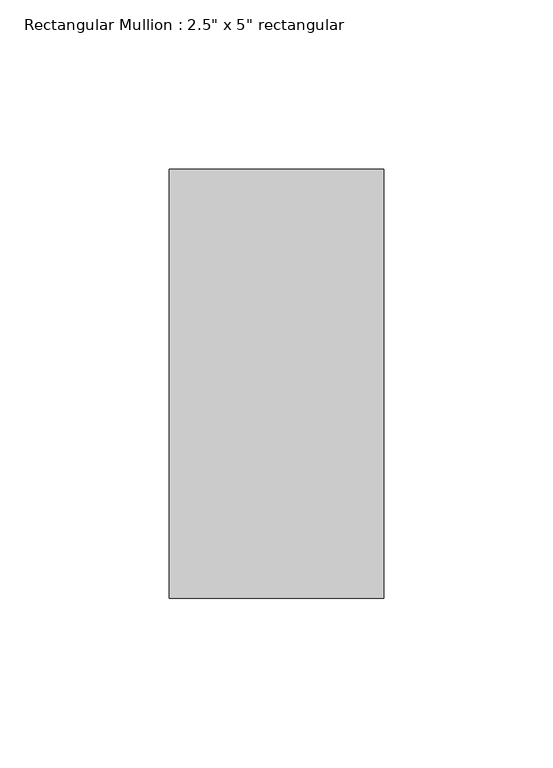
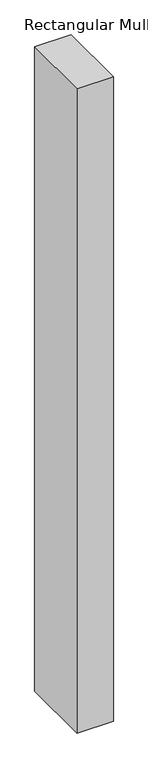
"""IFC4 building model written with IfcOpenShell, lengths in millimetres: member geometry."""

from ifc_helpers import new_model, si_unit, frame, origin, place, context, project, spatial, polyline, outline, extrude, source, transform, mapped, element, save


def member_7df25b28(model_context):
    return source(origin(), model_context, "Body", "SweptSolid", [
        extrude(outline(polyline([(0.0, 63.5), (0.0, -63.5), (-63.5, -63.5), (-63.5, 63.5), (0.0, 63.5)])), frame((0.0, 0.0, -1185.3333333), z_axis=(0.0, 0.0, 1.0), x_axis=(1.0, 0.0, 0.0)), (0.0, 0.0, 1.0), 1185.3333333),
    ])


if __name__ == "__main__":
    model = new_model("IFC4")
    model_context = context("Model", 3, world=origin())
    ifc_project = project(units=[si_unit("LENGTHUNIT", "METRE", prefix="MILLI")], contexts=[model_context])
    site = spatial("IfcSite", under=ifc_project)
    building = spatial("IfcBuilding", under=site)
    placement = place(None, origin())
    member_shape = member_7df25b28(model_context)
    element("IfcMember", 1, ObjectType="Rectangular Mullion : 2.5\" x 5\" rectangular", at=placement, inside=building, context=model_context, shape_type="MappedRepresentation", body=[
        mapped(member_shape, transform((0.0, 0.0, 0.0), x_axis=(1.0, 0.0, 0.0), y_axis=(0.0, 1.0, 0.0), z_axis=(0.0, 0.0, 1.0))),
    ])
    save(model, "model.ifc")

# Revit data of these elements
# Type "Rectangular Mullion : 2.5\" x 5\" rectangular"
#   built-in parameter 1007304 = 0.416667 (stored number, unit not read)
#   built-in parameter 1007301 = 0.104167 (stored number, unit not read)
#   built-in parameter 1007300 = 0.104167 (stored number, unit not read)
# Element 1 (IfcMember, "Rectangular Mullion : 2.5\" x 5\" rectangular")
#   Materials on its faces: "Aluminum"
# Materials
#   "Aluminum": class "Metal", colour RGB 247 247 247, transparency 0, Description = "Aluminum 6061", Cost = 0
